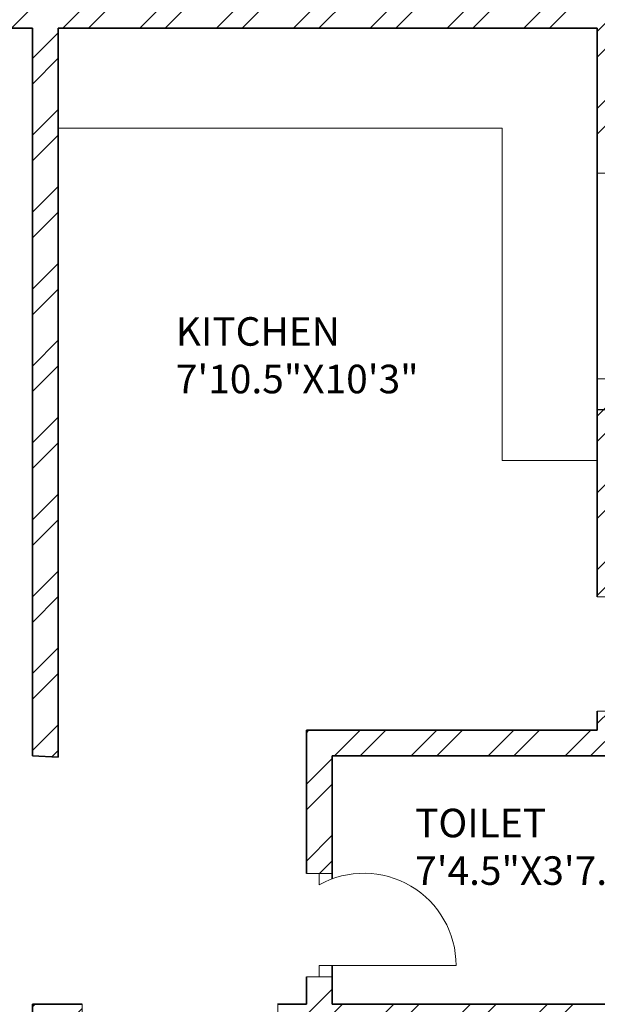
# Model space of a CAD drawing. Units: inches. Extents: x 2120 to 4013, y 1390 to 3019.
# Tile 24 of 59: x 2857 to 2959, y 1792 to 1964. Entities that reach past the tile are written whole.
import ezdxf

# ---------------------------------------------------------------- set-up
doc = ezdxf.new("R2010")
doc.units = ezdxf.units.IN
for name, color, linetype, lineweight in [('A-ANNO-DIMS', 2, 'Continuous', 18), ('A-AREA-IDEN', 7, 'Continuous', 18), ('A-DOOR', 3, 'Continuous', 18), ('A-FLOR-CASE', 8, 'Continuous', 18), ('A-GLAZ', 4, 'Continuous', 18), ('A-WALL', 7, 'Continuous', 35), ('A-WALL-PATT', 252, 'Continuous', 13)]:
    doc.layers.add(name, color=color, linetype=linetype, lineweight=lineweight)
doc.styles.get("Standard").update_dxf_attribs({"font": 'arial.ttf'})
doc.dimstyles.get("Standard").update_dxf_attribs({"dimtxt": 0.18, "dimasz": 0.18, "dimexe": 0.18, "dimexo": 0.0625, "dimgap": 0.09, "dimtad": 0, "dimtih": 1, "dimtoh": 1, "dimdec": 4, "dimzin": 0, "dimdsep": 46, "dimtxsty": 'Standard', "dimcen": 0.09, "dimadec": 0, "dimazin": 0, "dimtfac": 1, "dimtdec": 4, "dimtofl": 0, "dimtmove": 0, "dimatfit": 3, "dimfxl": 1, "dimtolj": 1, "dimtzin": 0, "dimarcsym": 0})

# ---------------------------------------------------------------- blocks, each defined once
blk = doc.blocks.new('DOOR-SWING-24IN-119p01DEG')
for p, q in [((0, 18.13), (4.5, 18.13)), ((4.5, 18.13), (2.25, 18.13)), ((2.25, 18.13), (2.25, 16.13)), ((2.25, 0), (2.25, 2)), ((2.25, 2), (26.25, 2)), ((0, 0), (4.5, 0)), ((4.5, 0), (2.25, 0))]:
    blk.add_line(p, q)
blk.add_arc((10.09, 2), 16.16, 0, 119.0137)
blk = doc.blocks.new('DOOR-SWING-24IN-112p55DEG')
for p, q in [((0, 20.02), (4.5, 20.02)), ((4.5, 20.02), (2.25, 20.02)), ((2.25, 20.02), (2.25, 18.02)), ((2.25, 0), (2.25, 2)), ((2.25, 2), (26.25, 2)), ((0, 0), (4.5, 0)), ((4.5, 0), (2.25, 0))]:
    blk.add_line(p, q)
blk.add_arc((8.9, 2), 17.35, 0, 112.5501)
blk = doc.blocks.new('DOOR-SWING-36IN-99p84DEG')
for p, q in [((0, 38.25), (0, 33.75)), ((0, 33.75), (0, 38.25)), ((0, 38.25), (0, 36)), ((34.3, 38.25), (34.3, 33.75)), ((0, 36), (2, 36)), ((2, 36), (2, 0)), ((34.3, 36), (32.3, 36)), ((34.3, 33.75), (34.3, 36))]:
    blk.add_line(p, q)
blk.add_arc((2, 30.75), 30.75, 270, 9.8355)
blk = doc.blocks.new('WIN-PLAN-36IN-02')
for p, q in [((2.25, 36), (0, 36)), ((0, 36), (4.5, 36)), ((2.25, 0), (2.25, 36)), ((0, 0), (4.5, 0)), ((4.5, 0), (2.25, 0))]:
    blk.add_line(p, q)
blk = doc.blocks.new('*D180')
at = {"layer": 'A-ANNO-DIMS', "color": 0, "lineweight": -2, "transparency": 16777216}
for p, q in [((2958.73, 1901.03), (2958.73, 1895.51)), ((2963.23, 1901.03), (2963.23, 1895.51)), ((2958.91, 1895.69), (2960.52, 1895.69)), ((2963.05, 1895.69), (2961.44, 1895.69))]:
    blk.add_line(p, q, dxfattribs=at)
at = {"layer": 'A-ANNO-DIMS', "color": 0, "transparency": 16777216}
for points in [[(2958.91, 1895.72), (2958.91, 1895.66), (2958.73, 1895.69)], [(2963.05, 1895.72), (2963.05, 1895.66), (2963.23, 1895.69)]]:
    blk.add_solid(points, dxfattribs=at)
at = {"layer": 'Defpoints', "color": 0, "transparency": 16777216}
for p in [(2958.73, 1901.09), (2963.23, 1901.09), (2963.23, 1895.69)]:
    blk.add_point(p, dxfattribs=at)
at = {"layer": 'A-ANNO-DIMS', "color": 0, "transparency": 16777216, "insert": (2960.98, 1895.69), "char_height": 0.18, "attachment_point": 5}
blk.add_mtext('\\A1;5 TYP.', dxfattribs=at)

msp = doc.modelspace()

# ---------------------------------------------------------------- hatches: boundary and pattern name
at = {"layer": 'A-WALL-PATT'}
h = msp.add_hatch(dxfattribs=at)
h.set_pattern_fill('ANSI32', color=256)
h.paths.add_polyline_path([(2271.7331, 2343.531), (2283.3788, 2343.531), (2283.3788, 2348.031), (2283.3788, 2352.5306), (2262.7331, 2352.5306), (2262.7331, 2182.638), (2267.2331, 2182.638), (2271.7331, 2182.638), (2271.7331, 2219.031), (2391.7331, 2219.031), (2391.7331, 2214.189), (2393.9831, 2214.189), (2396.2331, 2214.189), (2396.2331, 2219.031), (2420.2331, 2219.031), (2420.2331, 2225.7535), (2417.2197, 2225.7535), (2415.7331, 2225.7535), (2415.7331, 2223.5306), (2271.7331, 2223.5306)])
h.paths.add_polyline_path([(2380.0942, 2352.5306), (2343.3788, 2352.5306), (2343.3788, 2343.531), (2363.2331, 2343.531), (2363.2331, 2288.8489), (2365.4831, 2288.8489), (2367.7331, 2288.8489), (2367.7331, 2343.531), (2380.0942, 2343.531)], flags=17)
h.paths.add_polyline_path([(2432.4339, 2352.5306), (2404.0943, 2352.5306), (2404.0943, 2343.531), (2415.7331, 2343.531), (2415.7331, 2264.0306), (2367.7331, 2264.0306), (2367.7331, 2266.4872), (2363.2331, 2266.4872), (2363.2331, 2259.531), (2367.7331, 2259.531), (2415.7331, 2259.531), (2415.7331, 2255.0658), (2420.2331, 2255.0658), (2420.2331, 2259.531), (2424.5717, 2259.531), (2424.5717, 2261.781), (2424.5717, 2264.0306), (2420.2331, 2264.0306), (2420.2331, 2343.531), (2432.4339, 2343.531)])
h.paths.add_polyline_path([(2508.9115, 2352.5306), (2456.4339, 2352.5306), (2456.4339, 2343.531), (2468.2331, 2343.531), (2468.2331, 2264.0306), (2448.0487, 2264.0306), (2448.0487, 2259.531), (2468.2331, 2259.531), (2468.2331, 2255.5496), (2472.7331, 2255.5496), (2472.7331, 2343.531), (2508.9115, 2343.531)])
h.paths.add_polyline_path([(2637.7331, 2352.5306), (2544.9116, 2352.5306), (2544.9116, 2343.531), (2589.7331, 2343.531), (2633.2331, 2343.531), (2637.7331, 2343.531)])
h.paths.add_polyline_path([(2594.2331, 2343.5306), (2589.7331, 2343.5306), (2589.7331, 2259.5306), (2589.7331, 2252.4915), (2591.9831, 2252.4915), (2594.2331, 2252.4915)])
h.paths.add_polyline_path([(2637.7331, 2223.5306), (2594.2331, 2223.5306), (2594.2331, 2230.1988), (2591.9831, 2230.1988), (2589.7331, 2230.1988), (2589.7331, 2223.5306), (2472.7331, 2223.5306), (2468.2331, 2223.5306), (2468.2331, 2219.031), (2628.7331, 2219.031), (2628.7331, 2138.031), (2637.7331, 2138.031)])
h.paths.add_polyline_path([(3822.6535, 2458.4402), (3874.9468, 2458.4402), (3874.9468, 2476.9866), (3822.6535, 2476.9866)], flags=9)
h.paths.add_polyline_path([(3834.6921, 2781.8174), (3935.9206, 2781.8174), (3935.9206, 2800.3638), (3834.6921, 2800.3638)], flags=9)
h.paths.add_polyline_path([(3832.2843, 2837.9683), (3884.5776, 2837.9683), (3884.5776, 2856.5146), (3832.2843, 2856.5146)], flags=9)
h.paths.add_polyline_path([(3830.9388, 2861.4782), (3956.8958, 2861.4782), (3956.8958, 2880.0245), (3830.9388, 2880.0245)], flags=9)
h.paths.add_polyline_path([(3870.6966, 2352.5752), (3887.9272, 2352.5752), (3887.9272, 2377.3037), (3870.6966, 2377.3037)], flags=9)
h.paths.add_polyline_path([(3289.2701, 2413.161), (3435.2223, 2413.161), (3435.2223, 2450.2538), (3289.2701, 2450.2538)], flags=9)
h.paths.add_polyline_path([(2487.6944, 2414.3601), (2637.8335, 2414.3601), (2637.8335, 2451.4528), (2487.6944, 2451.4528)], flags=9)
h.paths.add_polyline_path([(2567.3724, 1457.9199), (2815.296, 1457.9199), (2815.296, 1495.0127), (2567.3724, 1495.0127)], flags=9)
h.paths.add_polyline_path([(2655.3825, 2093.2363), (2685.9555, 2093.2363), (2685.9555, 2111.8937), (2655.3825, 2111.8937)], flags=9)
h.paths.add_polyline_path([(2543.9218, 1550.6671), (2587.8406, 1550.6671), (2587.8406, 1569.3244), (2543.9218, 1569.3244)], flags=9)
h.paths.add_polyline_path([(2905.1384, 1543.8113), (2949.0572, 1543.8113), (2949.0572, 1562.4686), (2905.1384, 1562.4686)], flags=9)
h.paths.add_polyline_path([(2736.4118, 1702.4736), (2784.2153, 1702.4736), (2784.2153, 1721.1309), (2736.4118, 1721.1309)], flags=9)
h.paths.add_polyline_path([(2912.8666, 1710.4168), (2951.707, 1710.4168), (2951.707, 1729.0741), (2912.8666, 1729.0741)], flags=9)
h.paths.add_polyline_path([(2923.5785, 1763.5038), (2959.7279, 1763.5038), (2959.7279, 1782.1611), (2923.5785, 1782.1611)], flags=9)
h.paths.add_polyline_path([(2925.2114, 1809.6137), (2967.1861, 1809.6137), (2967.1861, 1828.271), (2925.2114, 1828.271)], flags=9)
h.paths.add_polyline_path([(2996.2711, 1878.9003), (2996.2711, 1913.109), (2977.6138, 1913.109), (2977.6138, 1878.9003)], flags=9)
h.paths.add_polyline_path([(2883.0859, 1895.7192), (2927.1855, 1895.7192), (2927.1855, 1914.3766), (2883.0859, 1914.3766)], flags=9)
h.paths.add_polyline_path([(2787.3924, 1810.8013), (2841.0213, 1810.8013), (2841.0213, 1829.4587), (2787.3924, 1829.4587)], flags=9)
h.paths.add_polyline_path([(2775.6399, 2101.7395), (2829.2689, 2101.7395), (2829.2689, 2120.3968), (2775.6399, 2120.3968)], flags=9)
h.paths.add_polyline_path([(2913.0263, 2075.817), (2951.8667, 2075.817), (2951.8667, 2094.4744), (2913.0263, 2094.4744)], flags=9)
h.paths.add_polyline_path([(2929.966, 2133.3669), (2966.1154, 2133.3669), (2966.1154, 2152.0243), (2929.966, 2152.0243)], flags=9)
h.paths.add_polyline_path([(2932.7502, 2182.6088), (2968.8996, 2182.6088), (2968.8996, 2201.2662), (2932.7502, 2201.2662)], flags=9)
h.paths.add_polyline_path([(2996.0681, 2266.3173), (2996.0681, 2300.5261), (2977.4108, 2300.5261), (2977.4108, 2266.3173)], flags=9)
h.paths.add_polyline_path([(2885.1039, 2279.2186), (2929.2035, 2279.2186), (2929.2035, 2297.8759), (2885.1039, 2297.8759)], flags=9)
h.paths.add_polyline_path([(2735.7042, 2218.3197), (2783.5078, 2218.3197), (2783.5078, 2236.9771), (2735.7042, 2236.9771)], flags=9)
h.paths.add_polyline_path([(2635.6049, 2044.0085), (2648.9678, 2044.0085), (2648.9678, 2054.312), (2635.6049, 2054.312)], flags=9)
h.paths.add_polyline_path([(2714.0148, 1923.0473), (2727.3777, 1923.0473), (2727.3777, 1933.3508), (2714.0148, 1933.3508)], flags=9)
h.paths.add_polyline_path([(2709.0345, 1988.1628), (2722.3974, 1988.1628), (2722.3974, 1998.4663), (2709.0345, 1998.4663)], flags=9)
h.paths.add_polyline_path([(2592.8935, 1962.1763), (2606.2564, 1962.1763), (2606.2564, 1972.4799), (2592.8935, 1972.4799)], flags=9)
h.paths.add_polyline_path([(2618.3996, 1985.9724), (2644.1942, 1985.9724), (2644.1942, 1996.2759), (2618.3996, 1996.2759)], flags=9)
h.paths.add_polyline_path([(2601.279, 1920.5869), (2614.6419, 1920.5869), (2614.6419, 1930.8904), (2601.279, 1930.8904)], flags=9)
h.paths.add_polyline_path([(2692.3278, 1932.7645), (2704.5311, 1932.7645), (2704.5311, 1943.0681), (2692.3278, 1943.0681)], flags=9)
h.paths.add_polyline_path([(2311.122, 1672.7318), (2355.0408, 1672.7318), (2355.0408, 1691.3892), (2311.122, 1691.3892)], flags=9)
h.paths.add_polyline_path([(2456.2551, 1632.3198), (2492.4796, 1632.3198), (2492.4796, 1650.9772), (2456.2551, 1650.9772)], flags=9)
h.paths.add_polyline_path([(2401.0766, 1631.4793), (2437.301, 1631.4793), (2437.301, 1650.1367), (2401.0766, 1650.1367)], flags=9)
h.paths.add_polyline_path([(2546.7054, 1700.9235), (2594.509, 1700.9235), (2594.509, 1719.5809), (2546.7054, 1719.5809)], flags=9)
h.paths.add_polyline_path([(2445.4866, 1766.9937), (2497.5261, 1766.9937), (2497.5261, 1785.651), (2445.4866, 1785.651)], flags=9)
h.paths.add_polyline_path([(2287.9992, 1739.7675), (2326.8396, 1739.7675), (2326.8396, 1758.4248), (2287.9992, 1758.4248)], flags=9)
h.paths.add_polyline_path([(2458.5279, 1924.7607), (2510.5675, 1924.7607), (2510.5675, 1943.4181), (2458.5279, 1943.4181)], flags=9)
h.paths.add_polyline_path([(2309.2811, 1902.7642), (2345.4305, 1902.7642), (2345.4305, 1921.4215), (2309.2811, 1921.4215)], flags=9)
h.paths.add_polyline_path([(2490.7554, 2018.9392), (2530.7896, 2018.9392), (2530.7896, 2037.5965), (2490.7554, 2037.5965)], flags=9)
h.paths.add_polyline_path([(2402.143, 2024.7393), (2438.5414, 2024.7393), (2438.5414, 2043.3966), (2402.143, 2043.3966)], flags=9)
h.paths.add_polyline_path([(2287.856, 1931.7926), (2326.6964, 1931.7926), (2326.6964, 1950.4499), (2287.856, 1950.4499)], flags=9)
h.paths.add_polyline_path([(2281.7979, 2193.5771), (2320.6383, 2193.5771), (2320.6383, 2212.2344), (2281.7979, 2212.2344)], flags=25)
h.paths.add_polyline_path([(2484.0754, 2093.892), (2536.115, 2093.892), (2536.115, 2112.5494), (2484.0754, 2112.5494)], flags=9)
h.paths.add_polyline_path([(2624.7948, 2281.8639), (2624.7948, 2311.4137), (2606.1375, 2311.4137), (2606.1375, 2281.8639)], flags=9)
h.paths.add_polyline_path([(2507.5036, 2290.3639), (2541.934, 2290.3639), (2541.934, 2309.0212), (2507.5036, 2309.0212)], flags=9)
h.paths.add_polyline_path([(2423.1076, 2285.2202), (2459.332, 2285.2202), (2459.332, 2303.8776), (2423.1076, 2303.8776)], flags=9)
h.paths.add_polyline_path([(2374.5467, 2289.6272), (2410.7711, 2289.6272), (2410.7711, 2308.2846), (2374.5467, 2308.2846)], flags=25)
h.paths.add_polyline_path([(2277.4907, 2227.5651), (2316.3311, 2227.5651), (2316.3311, 2246.2224), (2277.4907, 2246.2224)], flags=25)
h.paths.add_polyline_path([(2655.3825, 2093.2367), (2685.9555, 2093.2367), (2685.9555, 2111.894), (2655.3825, 2111.894)], flags=9)
h.paths.add_polyline_path([(2543.9217, 1550.6674), (2587.8406, 1550.6674), (2587.8406, 1569.3247), (2543.9217, 1569.3247)], flags=9)
h.paths.add_polyline_path([(2905.1384, 1543.8116), (2949.0572, 1543.8116), (2949.0572, 1562.4689), (2905.1384, 1562.4689)], flags=9)
h.paths.add_polyline_path([(2736.4118, 1702.4739), (2784.2153, 1702.4739), (2784.2153, 1721.1312), (2736.4118, 1721.1312)], flags=9)
h.paths.add_polyline_path([(2912.8666, 1710.4171), (2951.707, 1710.4171), (2951.707, 1729.0744), (2912.8666, 1729.0744)], flags=9)
h.paths.add_polyline_path([(2923.5785, 1763.5041), (2959.7279, 1763.5041), (2959.7279, 1782.1614), (2923.5785, 1782.1614)], flags=9)
h.paths.add_polyline_path([(2925.2114, 1809.614), (2967.1861, 1809.614), (2967.1861, 1828.2713), (2925.2114, 1828.2713)], flags=9)
h.paths.add_polyline_path([(2996.2711, 1878.9006), (2996.2711, 1913.1094), (2977.6137, 1913.1094), (2977.6137, 1878.9006)], flags=9)
h.paths.add_polyline_path([(2883.0859, 1895.7195), (2927.1855, 1895.7195), (2927.1855, 1914.3769), (2883.0859, 1914.3769)], flags=9)
h.paths.add_polyline_path([(2787.3924, 1810.8016), (2841.0213, 1810.8016), (2841.0213, 1829.459), (2787.3924, 1829.459)], flags=9)
h.paths.add_polyline_path([(2775.6399, 2101.7398), (2829.2688, 2101.7398), (2829.2688, 2120.3971), (2775.6399, 2120.3971)], flags=9)
h.paths.add_polyline_path([(2913.0263, 2075.8173), (2951.8667, 2075.8173), (2951.8667, 2094.4747), (2913.0263, 2094.4747)], flags=9)
h.paths.add_polyline_path([(2929.966, 2133.3672), (2966.1154, 2133.3672), (2966.1154, 2152.0246), (2929.966, 2152.0246)], flags=9)
h.paths.add_polyline_path([(2932.7502, 2182.6091), (2968.8996, 2182.6091), (2968.8996, 2201.2665), (2932.7502, 2201.2665)], flags=9)
h.paths.add_polyline_path([(2996.0681, 2266.3176), (2996.0681, 2300.5264), (2977.4108, 2300.5264), (2977.4108, 2266.3176)], flags=9)
h.paths.add_polyline_path([(2885.1039, 2279.2189), (2929.2035, 2279.2189), (2929.2035, 2297.8762), (2885.1039, 2297.8762)], flags=9)
h.paths.add_polyline_path([(2735.7042, 2218.32), (2783.5078, 2218.32), (2783.5078, 2236.9774), (2735.7042, 2236.9774)], flags=9)
h.paths.add_polyline_path([(2635.6048, 2044.0088), (2648.9677, 2044.0088), (2648.9677, 2054.3123), (2635.6048, 2054.3123)], flags=9)
h.paths.add_polyline_path([(2714.0148, 1923.0476), (2727.3777, 1923.0476), (2727.3777, 1933.3511), (2714.0148, 1933.3511)], flags=9)
h.paths.add_polyline_path([(2709.0345, 1988.1631), (2722.3974, 1988.1631), (2722.3974, 1998.4666), (2709.0345, 1998.4666)], flags=9)
h.paths.add_polyline_path([(2592.8935, 1962.1766), (2606.2564, 1962.1766), (2606.2564, 1972.4802), (2592.8935, 1972.4802)], flags=9)
h.paths.add_polyline_path([(2618.3995, 1985.9727), (2644.1942, 1985.9727), (2644.1942, 1996.2762), (2618.3995, 1996.2762)], flags=9)
h.paths.add_polyline_path([(2601.279, 1920.5872), (2614.6419, 1920.5872), (2614.6419, 1930.8908), (2601.279, 1930.8908)], flags=9)
h.paths.add_polyline_path([(2692.3278, 1932.7648), (2704.5311, 1932.7648), (2704.5311, 1943.0684), (2692.3278, 1943.0684)], flags=9)
h.paths.add_polyline_path([(2311.122, 1672.7321), (2355.0408, 1672.7321), (2355.0408, 1691.3895), (2311.122, 1691.3895)], flags=9)
h.paths.add_polyline_path([(2456.2551, 1632.3201), (2492.4795, 1632.3201), (2492.4795, 1650.9775), (2456.2551, 1650.9775)], flags=9)
h.paths.add_polyline_path([(2401.0766, 1631.4796), (2437.301, 1631.4796), (2437.301, 1650.137), (2401.0766, 1650.137)], flags=9)
h.paths.add_polyline_path([(2546.7054, 1700.9238), (2594.509, 1700.9238), (2594.509, 1719.5812), (2546.7054, 1719.5812)], flags=9)
h.paths.add_polyline_path([(2445.4866, 1766.994), (2497.5261, 1766.994), (2497.5261, 1785.6513), (2445.4866, 1785.6513)], flags=9)
h.paths.add_polyline_path([(2287.9992, 1739.7678), (2326.8396, 1739.7678), (2326.8396, 1758.4251), (2287.9992, 1758.4251)], flags=9)
h.paths.add_polyline_path([(2458.5279, 1924.7611), (2510.5675, 1924.7611), (2510.5675, 1943.4184), (2458.5279, 1943.4184)], flags=9)
h.paths.add_polyline_path([(2309.2811, 1902.7645), (2345.4305, 1902.7645), (2345.4305, 1921.4218), (2309.2811, 1921.4218)], flags=9)
h.paths.add_polyline_path([(2490.7554, 2018.9395), (2530.7895, 2018.9395), (2530.7895, 2037.5968), (2490.7554, 2037.5968)], flags=9)
h.paths.add_polyline_path([(2402.143, 2024.7396), (2438.5413, 2024.7396), (2438.5413, 2043.3969), (2402.143, 2043.3969)], flags=9)
h.paths.add_polyline_path([(2287.856, 1931.7929), (2326.6964, 1931.7929), (2326.6964, 1950.4502), (2287.856, 1950.4502)], flags=9)
h.paths.add_polyline_path([(2281.7979, 2193.5774), (2320.6383, 2193.5774), (2320.6383, 2212.2347), (2281.7979, 2212.2347)], flags=25)
h.paths.add_polyline_path([(2484.0754, 2093.8924), (2536.115, 2093.8924), (2536.115, 2112.5497), (2484.0754, 2112.5497)], flags=9)
h.paths.add_polyline_path([(2624.7948, 2281.8642), (2624.7948, 2311.414), (2606.1374, 2311.414), (2606.1374, 2281.8642)], flags=9)
h.paths.add_polyline_path([(2507.5035, 2290.3642), (2541.934, 2290.3642), (2541.934, 2309.0215), (2507.5035, 2309.0215)], flags=9)
h.paths.add_polyline_path([(2423.1075, 2285.2205), (2459.332, 2285.2205), (2459.332, 2303.8779), (2423.1075, 2303.8779)], flags=9)
h.paths.add_polyline_path([(2374.5467, 2289.6275), (2410.7711, 2289.6275), (2410.7711, 2308.2849), (2374.5467, 2308.2849)], flags=25)
h.paths.add_polyline_path([(2277.4907, 2227.5654), (2316.3311, 2227.5654), (2316.3311, 2246.2227), (2277.4907, 2246.2227)], flags=25)
h = msp.add_hatch(dxfattribs=at)
h.set_pattern_fill('ANSI32', color=256)
h.paths.add_polyline_path([(2271.7331, 1980.389), (2262.7331, 1980.389), (2262.7331, 1912.8434), (2267.2331, 1912.8434), (2271.7331, 1912.8434), (2271.7331, 1922.531), (2351.2331, 1922.531), (2351.2331, 1901.4728), (2355.7331, 1901.4728), (2355.7331, 1922.531), (2357.9815, 1922.531), (2357.9815, 1926.5306), (2271.7331, 1926.5306)])
h.paths.add_polyline_path([(2589.2331, 1949.1622), (2584.7331, 1949.1622), (2580.2331, 1949.1622), (2580.2331, 1874.5306), (2355.7331, 1874.5306), (2355.7331, 1880.1922), (2351.2331, 1880.1922), (2351.2331, 1874.5306), (2271.7331, 1874.5306), (2271.7331, 1888.8431), (2262.7331, 1888.8431), (2262.7331, 1842.2909), (2267.2331, 1842.2909), (2271.7331, 1842.2909), (2271.7331, 1865.531), (2415.7331, 1865.531), (2415.7331, 1779.7286), (2420.2331, 1779.7286), (2420.2331, 1865.531), (2589.2331, 1865.531)])
h.paths.add_polyline_path([(2271.7331, 1782.2906), (2262.7331, 1782.2906), (2262.7331, 1711.4639), (2267.2331, 1711.4639), (2271.7331, 1711.4639), (2271.7331, 1738.031), (2420.2331, 1738.031), (2420.2331, 1742.531), (2420.2331, 1747.3376), (2417.9831, 1747.3376), (2415.7331, 1747.3376), (2415.7331, 1742.5306), (2271.7331, 1742.5306)])
h.paths.add_polyline_path([(2271.7331, 1627.031), (2362.3957, 1627.031), (2362.3957, 1629.281), (2362.3957, 1631.5306), (2271.7331, 1631.5306), (2271.7331, 1675.4636), (2262.7331, 1675.4636), (2262.7331, 1581.531), (2405.3032, 1581.531), (2405.3032, 1586.031), (2405.3032, 1590.5306), (2396.2331, 1590.5306), (2396.2331, 1691.4513), (2418.7206, 1691.4513), (2418.7206, 1695.951), (2396.2331, 1695.951), (2391.7331, 1695.951), (2391.7331, 1631.5306), (2386.7425, 1631.5306), (2386.7425, 1629.2806), (2386.7425, 1627.031), (2391.7331, 1627.031), (2391.7331, 1586.1709), (2271.7331, 1586.1709)])
h.paths.add_polyline_path([(2459.6703, 1590.5306), (2429.3032, 1590.5306), (2429.3032, 1581.531), (2459.6703, 1581.531), (2459.6703, 1586.031)])
h.paths.add_polyline_path([(2501.2331, 1590.531), (2501.2331, 1665.0195), (2498.9831, 1665.0195), (2496.7331, 1665.0195), (2496.7331, 1590.5306), (2483.8201, 1590.5306), (2483.8201, 1590.1579), (2483.6704, 1590.1579), (2483.6704, 1581.531), (2505.0196, 1581.531), (2505.0196, 1583.781), (2505.0196, 1586.0306), (2501.2331, 1586.0306)])
h.paths.add_polyline_path([(2544.1361, 1583.781), (2544.1361, 1586.0306), (2527.1368, 1586.0306), (2527.1368, 1583.7806), (2527.1368, 1581.531), (2544.1361, 1581.531)])
h.paths.add_polyline_path([(3822.6535, 2458.4402), (3874.9468, 2458.4402), (3874.9468, 2476.9866), (3822.6535, 2476.9866)], flags=9)
h.paths.add_polyline_path([(3834.6921, 2781.8174), (3935.9206, 2781.8174), (3935.9206, 2800.3638), (3834.6921, 2800.3638)], flags=9)
h.paths.add_polyline_path([(3832.2843, 2837.9683), (3884.5776, 2837.9683), (3884.5776, 2856.5146), (3832.2843, 2856.5146)], flags=9)
h.paths.add_polyline_path([(3830.9388, 2861.4782), (3956.8958, 2861.4782), (3956.8958, 2880.0245), (3830.9388, 2880.0245)], flags=9)
h.paths.add_polyline_path([(3870.6966, 2352.5752), (3887.9272, 2352.5752), (3887.9272, 2377.3037), (3870.6966, 2377.3037)], flags=9)
h.paths.add_polyline_path([(3289.2701, 2413.161), (3435.2223, 2413.161), (3435.2223, 2450.2538), (3289.2701, 2450.2538)], flags=9)
h.paths.add_polyline_path([(2487.6944, 2414.3601), (2637.8335, 2414.3601), (2637.8335, 2451.4528), (2487.6944, 2451.4528)], flags=9)
h.paths.add_polyline_path([(2567.3724, 1457.9199), (2815.296, 1457.9199), (2815.296, 1495.0127), (2567.3724, 1495.0127)], flags=9)
h.paths.add_polyline_path([(2655.3825, 2093.2363), (2685.9555, 2093.2363), (2685.9555, 2111.8937), (2655.3825, 2111.8937)], flags=9)
h.paths.add_polyline_path([(2543.9218, 1550.6671), (2587.8406, 1550.6671), (2587.8406, 1569.3244), (2543.9218, 1569.3244)], flags=9)
h.paths.add_polyline_path([(2905.1384, 1543.8113), (2949.0572, 1543.8113), (2949.0572, 1562.4686), (2905.1384, 1562.4686)], flags=9)
h.paths.add_polyline_path([(2736.4118, 1702.4736), (2784.2153, 1702.4736), (2784.2153, 1721.1309), (2736.4118, 1721.1309)], flags=9)
h.paths.add_polyline_path([(2912.8666, 1710.4168), (2951.707, 1710.4168), (2951.707, 1729.0741), (2912.8666, 1729.0741)], flags=9)
h.paths.add_polyline_path([(2923.5785, 1763.5038), (2959.7279, 1763.5038), (2959.7279, 1782.1611), (2923.5785, 1782.1611)], flags=9)
h.paths.add_polyline_path([(2925.2114, 1809.6137), (2967.1861, 1809.6137), (2967.1861, 1828.271), (2925.2114, 1828.271)], flags=9)
h.paths.add_polyline_path([(2996.2711, 1878.9003), (2996.2711, 1913.109), (2977.6138, 1913.109), (2977.6138, 1878.9003)], flags=9)
h.paths.add_polyline_path([(2883.0859, 1895.7192), (2927.1855, 1895.7192), (2927.1855, 1914.3766), (2883.0859, 1914.3766)], flags=9)
h.paths.add_polyline_path([(2787.3924, 1810.8013), (2841.0213, 1810.8013), (2841.0213, 1829.4587), (2787.3924, 1829.4587)], flags=9)
h.paths.add_polyline_path([(2775.6399, 2101.7395), (2829.2689, 2101.7395), (2829.2689, 2120.3968), (2775.6399, 2120.3968)], flags=9)
h.paths.add_polyline_path([(2913.0263, 2075.817), (2951.8667, 2075.817), (2951.8667, 2094.4744), (2913.0263, 2094.4744)], flags=9)
h.paths.add_polyline_path([(2929.966, 2133.3669), (2966.1154, 2133.3669), (2966.1154, 2152.0243), (2929.966, 2152.0243)], flags=9)
h.paths.add_polyline_path([(2932.7502, 2182.6088), (2968.8996, 2182.6088), (2968.8996, 2201.2662), (2932.7502, 2201.2662)], flags=9)
h.paths.add_polyline_path([(2996.0681, 2266.3173), (2996.0681, 2300.5261), (2977.4108, 2300.5261), (2977.4108, 2266.3173)], flags=9)
h.paths.add_polyline_path([(2885.1039, 2279.2186), (2929.2035, 2279.2186), (2929.2035, 2297.8759), (2885.1039, 2297.8759)], flags=9)
h.paths.add_polyline_path([(2735.7042, 2218.3197), (2783.5078, 2218.3197), (2783.5078, 2236.9771), (2735.7042, 2236.9771)], flags=9)
h.paths.add_polyline_path([(2635.6049, 2044.0085), (2648.9678, 2044.0085), (2648.9678, 2054.312), (2635.6049, 2054.312)], flags=9)
h.paths.add_polyline_path([(2714.0148, 1923.0473), (2727.3777, 1923.0473), (2727.3777, 1933.3508), (2714.0148, 1933.3508)], flags=9)
h.paths.add_polyline_path([(2709.0345, 1988.1628), (2722.3974, 1988.1628), (2722.3974, 1998.4663), (2709.0345, 1998.4663)], flags=9)
h.paths.add_polyline_path([(2592.8935, 1962.1763), (2606.2564, 1962.1763), (2606.2564, 1972.4799), (2592.8935, 1972.4799)], flags=9)
h.paths.add_polyline_path([(2618.3996, 1985.9724), (2644.1942, 1985.9724), (2644.1942, 1996.2759), (2618.3996, 1996.2759)], flags=9)
h.paths.add_polyline_path([(2601.279, 1920.5869), (2614.6419, 1920.5869), (2614.6419, 1930.8904), (2601.279, 1930.8904)], flags=9)
h.paths.add_polyline_path([(2692.3278, 1932.7645), (2704.5311, 1932.7645), (2704.5311, 1943.0681), (2692.3278, 1943.0681)], flags=9)
h.paths.add_polyline_path([(2311.122, 1672.7318), (2355.0408, 1672.7318), (2355.0408, 1691.3892), (2311.122, 1691.3892)], flags=25)
h.paths.add_polyline_path([(2456.2551, 1632.3198), (2492.4796, 1632.3198), (2492.4796, 1650.9772), (2456.2551, 1650.9772)], flags=9)
h.paths.add_polyline_path([(2401.0766, 1631.4793), (2437.301, 1631.4793), (2437.301, 1650.1367), (2401.0766, 1650.1367)], flags=9)
h.paths.add_polyline_path([(2546.7054, 1700.9235), (2594.509, 1700.9235), (2594.509, 1719.5809), (2546.7054, 1719.5809)], flags=9)
h.paths.add_polyline_path([(2445.4866, 1766.9937), (2497.5261, 1766.9937), (2497.5261, 1785.651), (2445.4866, 1785.651)], flags=9)
h.paths.add_polyline_path([(2287.9992, 1739.7675), (2326.8396, 1739.7675), (2326.8396, 1758.4248), (2287.9992, 1758.4248)], flags=24)
h.paths.add_polyline_path([(2458.5279, 1924.7607), (2510.5675, 1924.7607), (2510.5675, 1943.4181), (2458.5279, 1943.4181)], flags=25)
h.paths.add_polyline_path([(2309.2811, 1902.7642), (2345.4305, 1902.7642), (2345.4305, 1921.4215), (2309.2811, 1921.4215)], flags=25)
h.paths.add_polyline_path([(2490.7554, 2018.9392), (2530.7896, 2018.9392), (2530.7896, 2037.5965), (2490.7554, 2037.5965)], flags=9)
h.paths.add_polyline_path([(2402.143, 2024.7393), (2438.5414, 2024.7393), (2438.5414, 2043.3966), (2402.143, 2043.3966)], flags=9)
h.paths.add_polyline_path([(2287.856, 1931.7926), (2326.6964, 1931.7926), (2326.6964, 1950.4499), (2287.856, 1950.4499)], flags=25)
h.paths.add_polyline_path([(2281.7979, 2193.5771), (2320.6383, 2193.5771), (2320.6383, 2212.2344), (2281.7979, 2212.2344)], flags=9)
h.paths.add_polyline_path([(2484.0754, 2093.892), (2536.115, 2093.892), (2536.115, 2112.5494), (2484.0754, 2112.5494)], flags=9)
h.paths.add_polyline_path([(2624.7948, 2281.8639), (2624.7948, 2311.4137), (2606.1375, 2311.4137), (2606.1375, 2281.8639)], flags=9)
h.paths.add_polyline_path([(2507.5036, 2290.3639), (2541.934, 2290.3639), (2541.934, 2309.0212), (2507.5036, 2309.0212)], flags=9)
h.paths.add_polyline_path([(2423.1076, 2285.2202), (2459.332, 2285.2202), (2459.332, 2303.8776), (2423.1076, 2303.8776)], flags=9)
h.paths.add_polyline_path([(2374.5467, 2289.6272), (2410.7711, 2289.6272), (2410.7711, 2308.2846), (2374.5467, 2308.2846)], flags=9)
h.paths.add_polyline_path([(2277.4907, 2227.5651), (2316.3311, 2227.5651), (2316.3311, 2246.2224), (2277.4907, 2246.2224)], flags=9)
h.paths.add_polyline_path([(2655.3825, 2093.2367), (2685.9555, 2093.2367), (2685.9555, 2111.894), (2655.3825, 2111.894)], flags=9)
h.paths.add_polyline_path([(2543.9217, 1550.6674), (2587.8406, 1550.6674), (2587.8406, 1569.3247), (2543.9217, 1569.3247)], flags=9)
h.paths.add_polyline_path([(2905.1384, 1543.8116), (2949.0572, 1543.8116), (2949.0572, 1562.4689), (2905.1384, 1562.4689)], flags=9)
h.paths.add_polyline_path([(2736.4118, 1702.4739), (2784.2153, 1702.4739), (2784.2153, 1721.1312), (2736.4118, 1721.1312)], flags=9)
h.paths.add_polyline_path([(2912.8666, 1710.4171), (2951.707, 1710.4171), (2951.707, 1729.0744), (2912.8666, 1729.0744)], flags=9)
h.paths.add_polyline_path([(2923.5785, 1763.5041), (2959.7279, 1763.5041), (2959.7279, 1782.1614), (2923.5785, 1782.1614)], flags=9)
h.paths.add_polyline_path([(2925.2114, 1809.614), (2967.1861, 1809.614), (2967.1861, 1828.2713), (2925.2114, 1828.2713)], flags=9)
h.paths.add_polyline_path([(2996.2711, 1878.9006), (2996.2711, 1913.1094), (2977.6137, 1913.1094), (2977.6137, 1878.9006)], flags=9)
h.paths.add_polyline_path([(2883.0859, 1895.7195), (2927.1855, 1895.7195), (2927.1855, 1914.3769), (2883.0859, 1914.3769)], flags=9)
h.paths.add_polyline_path([(2787.3924, 1810.8016), (2841.0213, 1810.8016), (2841.0213, 1829.459), (2787.3924, 1829.459)], flags=9)
h.paths.add_polyline_path([(2775.6399, 2101.7398), (2829.2688, 2101.7398), (2829.2688, 2120.3971), (2775.6399, 2120.3971)], flags=9)
h.paths.add_polyline_path([(2913.0263, 2075.8173), (2951.8667, 2075.8173), (2951.8667, 2094.4747), (2913.0263, 2094.4747)], flags=9)
h.paths.add_polyline_path([(2929.966, 2133.3672), (2966.1154, 2133.3672), (2966.1154, 2152.0246), (2929.966, 2152.0246)], flags=9)
h.paths.add_polyline_path([(2932.7502, 2182.6091), (2968.8996, 2182.6091), (2968.8996, 2201.2665), (2932.7502, 2201.2665)], flags=9)
h.paths.add_polyline_path([(2996.0681, 2266.3176), (2996.0681, 2300.5264), (2977.4108, 2300.5264), (2977.4108, 2266.3176)], flags=9)
h.paths.add_polyline_path([(2885.1039, 2279.2189), (2929.2035, 2279.2189), (2929.2035, 2297.8762), (2885.1039, 2297.8762)], flags=9)
h.paths.add_polyline_path([(2735.7042, 2218.32), (2783.5078, 2218.32), (2783.5078, 2236.9774), (2735.7042, 2236.9774)], flags=9)
h.paths.add_polyline_path([(2635.6048, 2044.0088), (2648.9677, 2044.0088), (2648.9677, 2054.3123), (2635.6048, 2054.3123)], flags=9)
h.paths.add_polyline_path([(2714.0148, 1923.0476), (2727.3777, 1923.0476), (2727.3777, 1933.3511), (2714.0148, 1933.3511)], flags=9)
h.paths.add_polyline_path([(2709.0345, 1988.1631), (2722.3974, 1988.1631), (2722.3974, 1998.4666), (2709.0345, 1998.4666)], flags=9)
h.paths.add_polyline_path([(2592.8935, 1962.1766), (2606.2564, 1962.1766), (2606.2564, 1972.4802), (2592.8935, 1972.4802)], flags=9)
h.paths.add_polyline_path([(2618.3995, 1985.9727), (2644.1942, 1985.9727), (2644.1942, 1996.2762), (2618.3995, 1996.2762)], flags=9)
h.paths.add_polyline_path([(2601.279, 1920.5872), (2614.6419, 1920.5872), (2614.6419, 1930.8908), (2601.279, 1930.8908)], flags=9)
h.paths.add_polyline_path([(2692.3278, 1932.7648), (2704.5311, 1932.7648), (2704.5311, 1943.0684), (2692.3278, 1943.0684)], flags=9)
h.paths.add_polyline_path([(2311.122, 1672.7321), (2355.0408, 1672.7321), (2355.0408, 1691.3895), (2311.122, 1691.3895)], flags=25)
h.paths.add_polyline_path([(2456.2551, 1632.3201), (2492.4795, 1632.3201), (2492.4795, 1650.9775), (2456.2551, 1650.9775)], flags=9)
h.paths.add_polyline_path([(2401.0766, 1631.4796), (2437.301, 1631.4796), (2437.301, 1650.137), (2401.0766, 1650.137)], flags=9)
h.paths.add_polyline_path([(2546.7054, 1700.9238), (2594.509, 1700.9238), (2594.509, 1719.5812), (2546.7054, 1719.5812)], flags=9)
h.paths.add_polyline_path([(2445.4866, 1766.994), (2497.5261, 1766.994), (2497.5261, 1785.6513), (2445.4866, 1785.6513)], flags=9)
h.paths.add_polyline_path([(2287.9992, 1739.7678), (2326.8396, 1739.7678), (2326.8396, 1758.4251), (2287.9992, 1758.4251)], flags=24)
h.paths.add_polyline_path([(2458.5279, 1924.7611), (2510.5675, 1924.7611), (2510.5675, 1943.4184), (2458.5279, 1943.4184)], flags=25)
h.paths.add_polyline_path([(2309.2811, 1902.7645), (2345.4305, 1902.7645), (2345.4305, 1921.4218), (2309.2811, 1921.4218)], flags=25)
h.paths.add_polyline_path([(2490.7554, 2018.9395), (2530.7895, 2018.9395), (2530.7895, 2037.5968), (2490.7554, 2037.5968)], flags=9)
h.paths.add_polyline_path([(2402.143, 2024.7396), (2438.5413, 2024.7396), (2438.5413, 2043.3969), (2402.143, 2043.3969)], flags=9)
h.paths.add_polyline_path([(2287.856, 1931.7929), (2326.6964, 1931.7929), (2326.6964, 1950.4502), (2287.856, 1950.4502)], flags=25)
h.paths.add_polyline_path([(2281.7979, 2193.5774), (2320.6383, 2193.5774), (2320.6383, 2212.2347), (2281.7979, 2212.2347)], flags=9)
h.paths.add_polyline_path([(2484.0754, 2093.8924), (2536.115, 2093.8924), (2536.115, 2112.5497), (2484.0754, 2112.5497)], flags=9)
h.paths.add_polyline_path([(2624.7948, 2281.8642), (2624.7948, 2311.414), (2606.1374, 2311.414), (2606.1374, 2281.8642)], flags=9)
h.paths.add_polyline_path([(2507.5035, 2290.3642), (2541.934, 2290.3642), (2541.934, 2309.0215), (2507.5035, 2309.0215)], flags=9)
h.paths.add_polyline_path([(2423.1075, 2285.2205), (2459.332, 2285.2205), (2459.332, 2303.8779), (2423.1075, 2303.8779)], flags=9)
h.paths.add_polyline_path([(2374.5467, 2289.6275), (2410.7711, 2289.6275), (2410.7711, 2308.2849), (2374.5467, 2308.2849)], flags=9)
h.paths.add_polyline_path([(2277.4907, 2227.5654), (2316.3311, 2227.5654), (2316.3311, 2246.2227), (2277.4907, 2246.2227)], flags=9)
h = msp.add_hatch(dxfattribs=at)
h.set_pattern_fill('ANSI32', color=256)
h.paths.add_polyline_path([(2271.7331, 2122.6377), (2262.7331, 2122.6377), (2262.7331, 2040.3893), (2267.2331, 2040.3893), (2271.7331, 2040.3893), (2271.7331, 2044.8856), (2271.7331, 2070.531), (2391.7331, 2070.531), (2391.7331, 1926.5306), (2388.3993, 1926.5306), (2388.3993, 1922.531), (2395.7331, 1922.531), (2395.7331, 1992.531), (2400.4511, 1992.531), (2400.4511, 1997.0306), (2395.7331, 1997.0306), (2395.7331, 2070.531), (2443.7331, 2070.531), (2443.7331, 2046.1368), (2448.2331, 2046.1368), (2448.2331, 2070.531), (2580.2331, 2070.531), (2580.2331, 1997.0306), (2492.9076, 1997.0306), (2492.9076, 1992.531), (2580.2331, 1992.531), (2580.2331, 1983.9368), (2589.2331, 1983.9368), (2589.2331, 2070.531), (2589.2331, 2075.0306), (2396.2331, 2075.0306), (2396.2331, 2184.3565), (2393.9831, 2184.3565), (2391.7331, 2184.3565), (2391.7331, 2075.0306), (2271.7331, 2075.0306)])
h.paths.add_polyline_path([(2724.7331, 2138.0306), (2628.7331, 2138.0306), (2628.7331, 2070.5306), (2628.7331, 2067.0987), (2633.2331, 2067.0987), (2637.7331, 2067.0987), (2637.7331, 2070.531), (2657.3413, 2070.531), (2657.3413, 2079.5306), (2637.7331, 2079.5306), (2637.7331, 2129.031), (2715.7331, 2129.031), (2715.7331, 2079.5306), (2698.0378, 2079.5306), (2698.0378, 2070.531), (2715.7331, 2070.531), (2715.7331, 2012.1531), (2720.2331, 2012.1531), (2724.7331, 2012.1531)])
h.paths.add_polyline_path([(2724.7331, 2213.031), (2831.3209, 2213.031), (2831.3209, 2215.281), (2831.3209, 2217.5306), (2724.7331, 2217.5306), (2724.7331, 2343.531), (2751.8755, 2343.531), (2751.8755, 2352.5306), (2715.7331, 2352.5306), (2715.7331, 2138.031), (2724.7331, 2138.031)])
h.paths.add_polyline_path([(2902.53, 2352.5306), (2811.8755, 2352.5306), (2811.8755, 2343.531), (2867.2331, 2343.531), (2867.2331, 2217.5306), (2863.6364, 2217.5306), (2863.6364, 2213.031), (2871.7331, 2213.031), (2871.7331, 2217.531), (2871.7331, 2343.531), (2902.53, 2343.531)])
h.paths.add_polyline_path([(3009.7331, 2352.5306), (2938.53, 2352.5306), (2938.53, 2343.531), (2966.2331, 2343.531), (2966.2331, 2242.3281), (2968.4831, 2242.3281), (2970.7331, 2242.3281), (2970.7331, 2343.531), (3009.7331, 2343.531)])
h.paths.add_polyline_path([(3009.7331, 2217.5306), (2970.7331, 2217.5306), (2970.7331, 2220.5422), (2968.4831, 2220.5422), (2966.2331, 2220.5422), (2966.2331, 2217.5306), (2911.7752, 2217.5306), (2907.7331, 2217.5306), (2907.7331, 2213.0306), (2907.7331, 2194.9663), (2912.2331, 2194.9663), (2912.2331, 2213.031), (2970.7331, 2213.031), (3000.7331, 2213.031), (3000.7331, 2205.523), (3009.7331, 2205.523)])
h.paths.add_polyline_path([(3009.7331, 2181.5227), (3000.7331, 2181.5227), (3000.7331, 2165.0306), (2912.2331, 2165.0306), (2912.2331, 2170.8202), (2907.7331, 2170.8202), (2907.7331, 2165.0306), (2899.5169, 2165.0306), (2899.5169, 2162.7806), (2899.5169, 2160.531), (2907.7331, 2160.531), (2907.7331, 2137.3432), (2912.2331, 2137.3432), (2912.2331, 2160.531), (3000.7331, 2160.531), (3000.7331, 2150.4993), (3009.7331, 2150.4993)])
h.paths.add_polyline_path([(3009.7331, 2126.499), (3005.2331, 2126.499), (3000.7331, 2126.499), (3000.7331, 2112.5306), (2912.2331, 2112.5306), (2912.2331, 2115.6036), (2907.7331, 2115.6036), (2907.7331, 2108.031), (3000.7331, 2108.031), (3000.7331, 2084.7256), (3009.7331, 2084.7256)], flags=17)
h.paths.add_polyline_path([(3009.7331, 1971.531), (3009.7331, 2024.7253), (3000.7331, 2024.7253), (3000.7331, 2006.4153), (3000.7331, 1971.5306), (2864.2331, 1971.5306), (2864.2331, 2160.531), (2868.0522, 2160.531), (2868.0522, 2165.0306), (2859.7331, 2165.0306), (2859.7331, 1971.5306), (2724.7331, 1971.5306), (2724.7331, 1977.7012), (2715.7331, 1977.7012), (2715.7331, 1962.5306), (2715.7331, 1950.9035), (2720.2331, 1950.9035), (2724.7331, 1950.9035), (2724.7331, 1962.531), (2855.2331, 1962.531), (2859.7331, 1962.531), (2859.7331, 1835.031), (2864.2331, 1834.8158), (2864.2331, 1962.531), (2958.7331, 1962.531), (2958.7331, 1937.0925), (2963.2331, 1937.0925), (2963.2331, 1962.531), (3000.7331, 1962.531), (3009.7331, 1962.531)])
h.paths.add_polyline_path([(2724.7331, 1728.531), (2822.7164, 1728.531), (2822.7164, 1733.0306), (2724.7331, 1733.0306), (2724.7331, 1779.3416), (2715.7331, 1779.3416), (2715.7331, 1581.531), (2753.02, 1581.531), (2753.02, 1586.031), (2753.02, 1590.5306), (2724.7331, 1590.5306)])
h.paths.add_polyline_path([(2864.2331, 1590.531), (2864.2331, 1787.031), (2868.4075, 1787.031), (2868.4075, 1791.5306), (2859.7331, 1791.5306), (2859.7331, 1739.0306), (2859.7331, 1733.0306), (2854.3125, 1733.0306), (2854.3125, 1728.531), (2859.7331, 1728.531), (2859.7331, 1590.5306), (2813.02, 1590.5306), (2813.02, 1581.531), (2868.4123, 1581.531), (2868.4123, 1583.781), (2868.4123, 1586.0306), (2864.2331, 1586.0306)])
h.paths.add_polyline_path([(3009.7331, 1754.6619), (3000.7331, 1754.6619), (3000.7331, 1739.0306), (2912.2331, 1739.0306), (2912.2331, 1742.2257), (2907.7331, 1742.2257), (2907.7331, 1739.0306), (2907.7331, 1734.531), (3000.7331, 1734.531), (3000.7331, 1590.5306), (3000.7331, 1586.0306), (2971.3921, 1586.0306), (2971.3921, 1581.531), (3009.7331, 1581.531)])
h.paths.add_polyline_path([(2911.3921, 1583.781), (2911.3921, 1586.0306), (2891.2138, 1586.0306), (2891.2138, 1581.531), (2911.3921, 1581.531)])
h.paths.add_polyline_path([(3009.7331, 1799.8422), (3000.7331, 1799.8422), (3000.7331, 1791.5306), (2912.2331, 1791.5306), (2912.2331, 1796.3264), (2909.9831, 1796.3264), (2907.7331, 1796.3264), (2907.7331, 1791.5306), (2902.7033, 1791.5306), (2902.7033, 1787.031), (2907.7331, 1787.031), (2907.7331, 1761.1622), (2912.2331, 1761.1622), (2912.2331, 1787.031), (3000.7331, 1787.031), (3000.7331, 1778.6622), (3009.7331, 1778.6622)])
h.paths.add_polyline_path([(3009.7331, 1839.5306), (2963.2331, 1839.5306), (2963.2331, 1842.8629), (2960.9831, 1842.8629), (2958.7331, 1842.8629), (2958.7331, 1839.5306), (2907.7331, 1839.5306), (2907.7331, 1814.4599), (2912.2331, 1814.4599), (2912.2331, 1835.031), (3000.7331, 1835.031), (3000.7331, 1823.8425), (3009.7331, 1823.8425), (3009.7331, 1835.031)])
h.paths.add_polyline_path([(2963.2331, 1901.0922), (2960.9831, 1901.0922), (2958.7331, 1901.0922), (2958.7331, 1862.8843), (2963.2331, 1862.8843)], flags=17)
h.paths.add_polyline_path([(2724.7331, 1891.9826), (2724.7331, 1914.3416), (2715.7331, 1914.3416), (2715.7331, 1783.8416), (2637.7331, 1783.8416), (2637.7331, 1914.3416), (2628.7331, 1914.3416), (2624.7701, 1914.3416), (2624.7701, 1909.8416), (2624.7701, 1905.3419), (2628.7331, 1905.3419), (2628.7331, 1876.9915), (2628.7331, 1779.3419), (2637.7331, 1779.3419), (2715.7331, 1779.3419), (2724.7331, 1779.3419), (2724.7331, 1835.031)])
h.paths.add_polyline_path([(2637.7331, 1731.531), (2637.7331, 1779.3416), (2628.7331, 1779.3416), (2628.7331, 1731.5306), (2589.2331, 1731.5306), (2535.9814, 1731.5306), (2496.7331, 1731.5306), (2496.7331, 1725.6876), (2498.9831, 1725.6876), (2501.2331, 1725.6876), (2501.2331, 1727.031), (2628.7331, 1727.031), (2628.7331, 1680.4203), (2628.7331, 1590.5306), (2628.7331, 1586.0306), (2604.1361, 1586.0306), (2604.1361, 1581.531), (2637.7331, 1581.531), (2637.7331, 1590.531)])

# ---------------------------------------------------------------- linework, layer by layer
at = {"layer": 'A-FLOR-CASE'}
for p, q in [((2864.2331, 1944.9893), (2942.0522, 1944.9893)), ((2864.2331, 1944.989), (2942.0522, 1944.989)), ((2942.0522, 1944.9893), (2942.0522, 1886.7683)), ((2942.0522, 1944.989), (2942.0522, 1886.768)), ((2942.0522, 1886.7683), (2958.7331, 1886.7683)), ((2942.0522, 1886.768), (2958.7331, 1886.768))]:
    msp.add_line(p, q, dxfattribs=at)
at = {"layer": 'A-WALL'}
for p, q in [((2859.7331, 1962.531), (2724.7331, 1962.531)), ((2859.7331, 1962.5306), (2724.7331, 1962.5306)), ((2859.7331, 1835.031), (2859.7331, 1962.531)), ((2859.7331, 1835.0306), (2859.7331, 1962.5306)), ((2864.2331, 1834.8158), (2864.2331, 1962.531)), ((2958.7331, 1962.531), (2864.2331, 1962.531)), ((2864.2331, 1834.8155), (2864.2331, 1962.5306)), ((2958.7331, 1962.5306), (2864.2331, 1962.5306)), ((2958.7331, 1862.8843), (2958.7331, 1962.531)), ((2958.7331, 1862.884), (2958.7331, 1962.5306)), ((2958.7331, 1839.531), (2958.7331, 1842.8632)), ((2958.7331, 1839.5306), (2958.7331, 1842.8629)), ((2859.7331, 1839.531), (2859.7331, 1835.031)), ((2859.7331, 1839.5306), (2859.7331, 1835.0306)), ((2907.7331, 1839.531), (2907.7331, 1814.4599)), ((2916.7331, 1839.531), (2907.7331, 1839.531)), ((2958.7331, 1839.531), (2907.7331, 1839.531)), ((2958.7331, 1839.5306), (2907.7331, 1839.5306)), ((2907.7331, 1839.5306), (2907.7331, 1814.4596)), ((2916.7331, 1839.5306), (2907.7331, 1839.5306)), ((2921.2331, 1839.531), (2916.7331, 1839.531)), ((2921.2331, 1839.5306), (2916.7331, 1839.5306)), ((2864.2331, 1834.8158), (2859.7331, 1835.031)), ((2864.2331, 1834.8155), (2859.7331, 1835.0306)), ((3000.7331, 1835.031), (2912.2331, 1835.031)), ((2912.2331, 1813.4911), (2912.2331, 1835.031)), ((3000.7331, 1835.0306), (2912.2331, 1835.0306)), ((2912.2331, 1813.4908), (2912.2331, 1835.0306)), ((2912.2331, 1791.531), (2912.2331, 1798.3267)), ((2912.2331, 1791.5306), (2912.2331, 1798.3264)), ((2907.7331, 1796.3267), (2907.7331, 1791.531)), ((2907.7331, 1796.3264), (2907.7331, 1791.5306)), ((2859.7331, 1739.031), (2859.7331, 1791.531)), ((2859.7331, 1791.531), (2868.4075, 1791.531)), ((2868.4075, 1791.531), (2859.7331, 1791.531)), ((2868.4076, 1791.5306), (2859.7331, 1791.5306)), ((2859.7331, 1739.0306), (2859.7331, 1791.5306)), ((2859.7331, 1791.5306), (2868.4076, 1791.5306)), ((2902.7033, 1791.531), (2907.7331, 1791.531)), ((2907.7331, 1791.531), (2902.7033, 1791.531)), ((2907.7331, 1791.5306), (2902.7033, 1791.5306)), ((2902.7033, 1791.5306), (2907.7331, 1791.5306)), ((3000.7331, 1791.531), (2912.2331, 1791.531)), ((3000.7331, 1791.5306), (2912.2331, 1791.5306))]:
    msp.add_line(p, q, dxfattribs=at)

# ---------------------------------------------------------------- block references
at = {"layer": 'A-DOOR'}
for name, p in [('DOOR-SWING-24IN-112p55DEG', (2958.7331, 1842.8632)), ('DOOR-SWING-24IN-112p55DEG', (2958.7331, 1842.8629)), ('DOOR-SWING-24IN-119p01DEG', (2907.7331, 1796.3267)), ('DOOR-SWING-24IN-119p01DEG', (2907.7331, 1796.3264)), ('DOOR-SWING-36IN-99p84DEG', (2868.4075, 1753.281))]:
    msp.add_blockref(name, p, dxfattribs=at)
at = {"layer": 'A-GLAZ'}
for p in [(2958.7331, 1901.0925), (2958.7331, 1901.0922)]:
    msp.add_blockref('WIN-PLAN-36IN-02', p, dxfattribs=at)

# ---------------------------------------------------------------- texts
at = {"layer": 'A-AREA-IDEN', "char_height": 5, "attachment_point": 1}
for s, width, insert in [('KITCHEN\\P7\'10.5"X10\'3"', 194.340028, (2884.8475, 1911.8888)), ('KITCHEN\\P7\'10.5"X10\'3"', 194.340028, (2884.8475, 1911.8885)), ('TOILET\\P7\'4.5"X3\'7.5"', 122.766551, (2926.7922, 1825.7867)), ('TOILET\\P7\'4.5"X3\'7.5"', 122.766551, (2926.7922, 1825.7864))]:
    msp.add_mtext_dynamic_manual_height_columns(s, width=width, gutter_width=12.5, heights=[0], dxfattribs=dict(at, insert=insert))

# ---------------------------------------------------------------- dimensions: what is measured, and where the dimension line sits
at = {"layer": 'A-ANNO-DIMS'}
dim = msp.add_linear_dim(base=(2963.2331222497, 1895.6925467185), p1=(2958.7331222497, 1901.0925467185), p2=(2963.2331222497, 1901.0925467185), text='<> TYP.', dimstyle='Standard', override={"dimdec": 0, "dimlfac": 1, "dimrnd": 0, "dimzin": 0, "dimdsep": 46, "dimlunit": 2}, dxfattribs=at)
dim.commit()
dim.dimension.update_dxf_attribs({"geometry": '*D180', "text_midpoint": (2960.9831222497, 1895.6925467185)})

doc.saveas('drawing.dxf')
